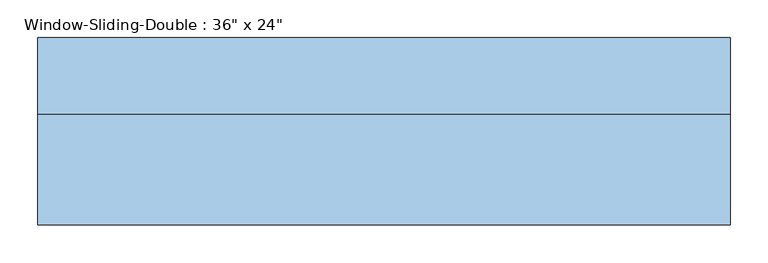
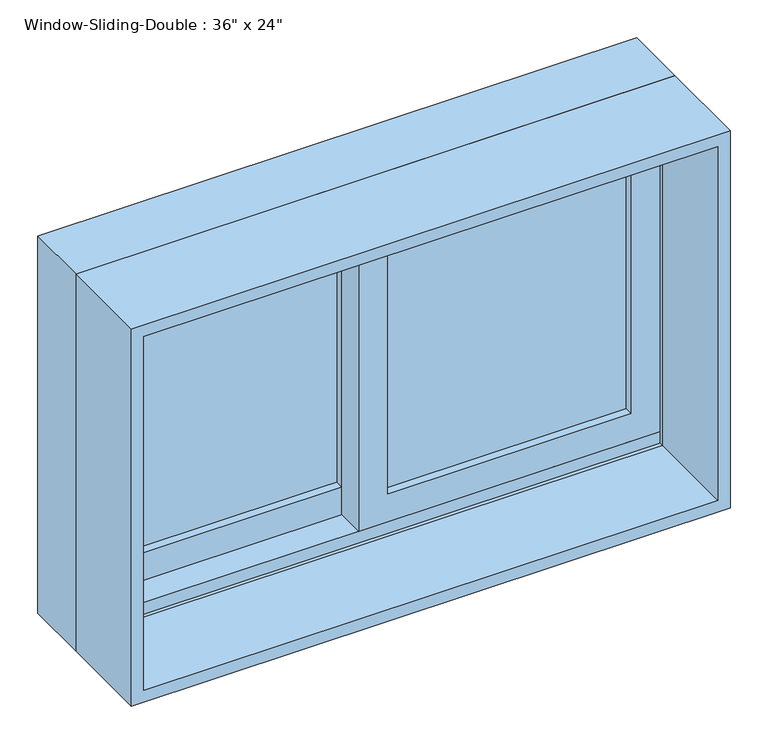
"""IFC4 building model written with IfcOpenShell, lengths in millimetres: window geometry."""

from ifc_helpers import new_model, si_unit, frame, origin, place, context, project, spatial, polyline, outline, extrude, faceted_brep, source, transform, mapped, element, save


def window_5ed62b27(model_context):
    return source(origin(), model_context, "Body", "SolidModel", [
        extrude(outline(polyline([(952.5, 438.15), (1504.95, 438.15), (1504.95, -22.225), (952.5, -22.225), (952.5, 438.15)]), holes=[polyline([(996.95, 22.225), (1460.5, 22.225), (1460.5, 393.7), (996.95, 393.7), (996.95, 22.225)])]), frame((0.0, 34.29, 0.0), z_axis=(0.0, 1.0, 0.0), x_axis=(0.0, 0.0, 1.0)), (0.0, 0.0, 1.0), 44.45),
        extrude(outline(polyline([(933.45, -438.15), (933.45, 22.225), (1504.95, 22.225), (1504.95, -438.15), (933.45, -438.15)]), holes=[polyline([(1460.5, -22.225), (996.95, -22.225), (996.95, -393.7), (1460.5, -393.7), (1460.5, -22.225)])]), frame((0.0, 78.74, 0.0), z_axis=(0.0, 1.0, 0.0), x_axis=(0.0, 0.0, 1.0)), (0.0, 0.0, 1.0), 44.45),
        extrude(outline(polyline([(-22.225, 110.49), (-22.225, 104.14), (-393.7, 104.14), (-393.7, 110.49), (-22.225, 110.49)])), frame((0.0, 0.0, 996.95), z_axis=(0.0, 0.0, 1.0), x_axis=(1.0, 0.0, 0.0)), (0.0, 0.0, 1.0), 463.55),
        extrude(outline(polyline([(-22.225, 97.79), (-22.225, 91.44), (-393.7, 91.44), (-393.7, 97.79), (-22.225, 97.79)])), frame((0.0, 0.0, 996.95), z_axis=(0.0, 0.0, 1.0), x_axis=(1.0, 0.0, 0.0)), (0.0, 0.0, 1.0), 463.55),
        extrude(outline(polyline([(393.7, 66.04), (393.7, 59.69), (22.225, 59.69), (22.225, 66.04), (393.7, 66.04)])), frame((0.0, 0.0, 996.95), z_axis=(0.0, 0.0, 1.0), x_axis=(1.0, 0.0, 0.0)), (0.0, 0.0, 1.0), 463.55),
        extrude(outline(polyline([(393.7, 53.34), (393.7, 46.99), (22.225, 46.99), (22.225, 53.34), (393.7, 53.34)])), frame((0.0, 0.0, 996.95), z_axis=(0.0, 0.0, 1.0), x_axis=(1.0, 0.0, 0.0)), (0.0, 0.0, 1.0), 463.55),
        extrude(outline(polyline([(1524.0, -457.2), (914.4, -457.2), (914.4, 457.2), (1524.0, 457.2), (1524.0, -457.2)]), holes=[polyline([(1504.95, 438.15), (933.45, 438.15), (933.45, -438.15), (1504.95, -438.15), (1504.95, 438.15)])]), frame((0.0, -118.11, 0.0), z_axis=(0.0, 1.0, 0.0), x_axis=(0.0, 0.0, 1.0)), (0.0, 0.0, 1.0), 146.05),
        faceted_brep([(-457.2, 27.94, 914.4), (-457.2, 129.54, 914.4), (457.2, 129.54, 914.4), (457.2, 27.94, 914.4), (-416.2778905, 129.54, 1483.0778905), (-416.2778905, 123.19, 1483.0778905), (-416.2778905, 123.19, 933.45), (-416.2778905, 129.54, 933.45), (416.2778905, 123.19, 1483.0778905), (416.2778905, 123.19, 933.45), (438.15, 123.19, 933.45), (438.15, 123.19, 1504.95), (-438.15, 123.19, 1504.95), (-438.15, 123.19, 933.45), (-438.15, 27.94, 1504.95), (-438.15, 27.94, 933.45), (-438.15, 34.29, 933.45), (-438.15, 34.29, 952.5), (-438.15, 78.74, 952.5), (-438.15, 78.74, 933.45), (457.2, 27.94, 1524.0), (-457.2, 27.94, 1524.0), (438.15, 27.94, 1504.95), (438.15, 27.94, 933.45), (-457.2, 129.54, 1524.0), (457.2, 129.54, 1524.0), (416.2778905, 129.54, 933.45), (416.2778905, 129.54, 1483.0778905), (438.15, 78.74, 933.45), (438.15, 78.74, 952.5), (438.15, 34.29, 952.5), (438.15, 34.29, 933.45)], [[[0, 1, 2, 3]], [[4, 5, 6, 7]], [[5, 8, 9, 10, 11, 12, 13, 6]], [[12, 14, 15, 16, 17, 18, 19, 13]], [[0, 3, 20, 21], [22, 23, 15, 14]], [[24, 1, 0, 21]], [[2, 1, 24, 25], [4, 7, 26, 27]], [[5, 4, 27, 8]], [[12, 11, 22, 14]], [[21, 20, 25, 24]], [[8, 27, 26, 9]], [[22, 11, 10, 28, 29, 30, 31, 23]], [[20, 3, 2, 25]], [[26, 7, 6, 13, 19, 28, 10, 9]], [[28, 19, 18, 29]], [[29, 18, 17, 30]], [[30, 17, 16, 31]], [[15, 23, 31, 16]]]),
    ])


if __name__ == "__main__":
    model = new_model("IFC4")
    model_context = context("Model", 3, world=origin())
    ifc_project = project(units=[si_unit("LENGTHUNIT", "METRE", prefix="MILLI")], contexts=[model_context])
    site = spatial("IfcSite", under=ifc_project)
    building = spatial("IfcBuilding", under=site)
    placement = place(None, origin())
    window_shape = window_5ed62b27(model_context)
    element("IfcWindow", 1, ObjectType="Window-Sliding-Double : 36\" x 24\"", at=placement, inside=building, context=model_context, shape_type="MappedRepresentation", body=[
        mapped(window_shape, transform((0.0, 0.0, 0.0), x_axis=(1.0, 0.0, 0.0), y_axis=(0.0, 1.0, 0.0), z_axis=(0.0, 0.0, 1.0))),
    ])
    save(model, "model.ifc")

# Revit data of these elements
# Type "Window-Sliding-Double : 36\" x 24\""
#   Type Mark = "27"
#   Fire Rating = "0.5h"
#   Assembly Code = "B2020100"
#   Analytic Construction = "Double glazing - domestic"
#   Window Inset [instance default] = 0' - 0"
#   Wall Thickness [instance default] = 0' - 6"
#   Visual Light Transmittance = 0.81
#   Thermal Resistance (R) = 1.8146 (h·ft²·°F)/BTU
#   Solar Heat Gain Coefficient = 0.76
#   Muntin Width = 1' - 2 5/8"
#   Muntin Height = 1' - 6 1/4"
#   Interior Wall Closure [instance default] = 0' - 2 3/4"
#   Heat Transfer Coefficient (U) = 0.5511 BTU/(h·ft²·°F)
#   Frame Extension [instance default] = 0' - 0 1/4"
#   Exterior Wall Closure [instance default] = 0' - 1 1/4"
#   Rough Width = 3' - 0 1/2"
#   Rough Height = 2' - 0 1/2"
#   Height = 2' - 0"
#   Extension Jamb [instance default] = 0' - 2 3/4"
#   Default Sill Height = 3' - 0"
#   Width = 3' - 0"
#   Interior Trim Visibility [instance default] = yes
#   Indicator Visibility [instance default] = yes
#   Exterior Trim Visibility [instance default] = yes
#   Muntin Visibility = yes
#   Extension Jamb Visibility [instance default] = yes
#   Muntin Pattern = Muntin Pattern_2x2 : Muntin Pattern_2x2
#   Interior Trim Material = Wood - Stained
#   Interior Trim = Trim-Window-Interior-Flat : Picture Frame
#   Interior Frame Material = Wood - Stained
#   Glass Panel Material = Glass
#   Exterior Trim Material = Clad - White
#   Exterior Trim = Trim-Window-Exterior-Flat : with Sill
#   Exterior Frame Material = Clad - White
#   Wall Closure = (empty or 0)
# Element 1 (IfcWindow, "Window-Sliding-Double : 36\" x 24\"")
#   Wall Thickness = 0' - 9"
#   Extension Jamb = 0' - 5 3/4"
#   Materials on its faces: "Wood - Stained", "Glass", "Clad - White"
# Materials
#   "Wood - Stained": class "Wood", colour RGB 224 178 126, transparency 0, Cost = 0
#   "Glass": class "Glass", colour RGB 0 128 192, transparency 0.75, Description = "Soda Lime Glass", Cost = 0
#   "Clad - White": class "Wood", colour RGB 0 0 0, transparency 0, Cost = 0
